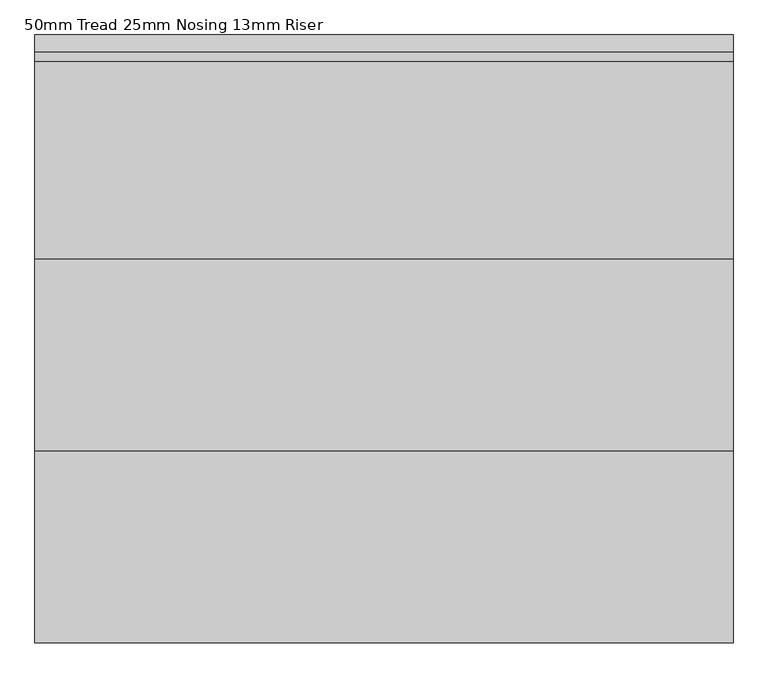
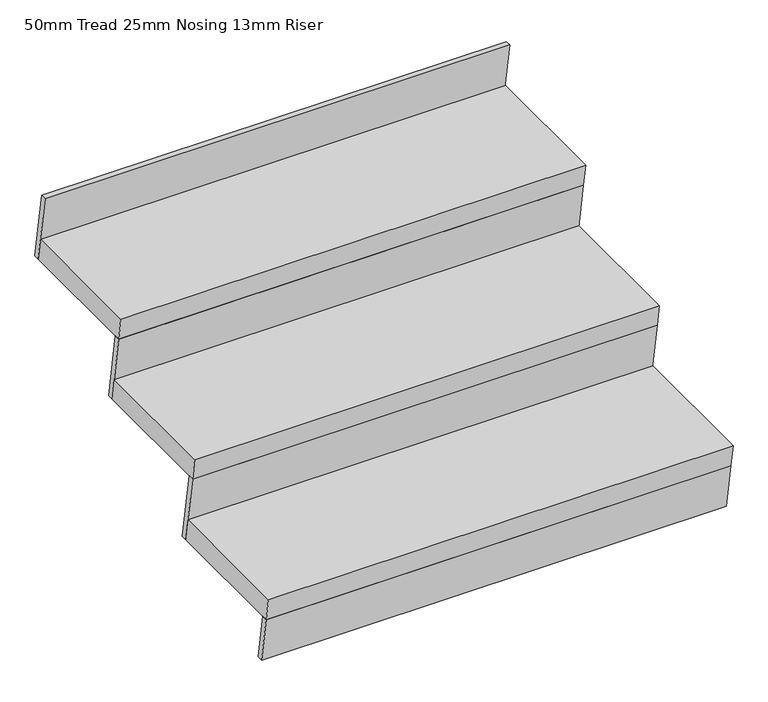
"""IFC4 building model written with IfcOpenShell, lengths in millimetres: stair flight geometry, 50mm Tread 25mm Nosing 13mm Riser."""

from ifc_helpers import new_model, si_unit, frame, origin, place, context, project, spatial, polyline, outline, extrude, source, transform, mapped, element, save


def stair_flight_50mm_tread_25mm_nosing_13mm_riser_f84e0c27(model_context):
    return source(origin(), model_context, "Body", "SweptSolid", [
        extrude(outline(polyline([(-5656.14356, -457.2), (-5356.14356, -457.2), (-5347.9414603, -507.2), (-5647.9414603, -507.2), (-5656.14356, -457.2)])), frame((-15773.6523905, 0.0, 0.0), z_axis=(1.0, 0.0, 0.0), x_axis=(0.0, 1.0, 0.0)), (0.0, 0.0, 1.0), 1000.0257813),
        extrude(outline(polyline([(-5647.9414603, -507.2), (-5635.2743907, -507.2), (-5618.4764904, -609.6), (-5631.14356, -609.6), (-5647.9414603, -507.2)])), frame((-15773.6523905, 0.0, 0.0), z_axis=(1.0, 0.0, 0.0), x_axis=(0.0, 1.0, 0.0)), (0.0, 0.0, 1.0), 1000.0257813),
        extrude(outline(polyline([(-5372.9414603, -354.8), (-5360.2743907, -354.8), (-5335.2743907, -507.2), (-5347.9414603, -507.2), (-5372.9414603, -354.8)])), frame((-15773.6523905, 0.0, 0.0), z_axis=(1.0, 0.0, 0.0), x_axis=(0.0, 1.0, 0.0)), (0.0, 0.0, 1.0), 1000.0257813),
        extrude(outline(polyline([(-5381.14356, -304.8), (-5081.14356, -304.8), (-5072.9414603, -354.8), (-5372.9414603, -354.8), (-5381.14356, -304.8)])), frame((-15773.6523905, 0.0, 0.0), z_axis=(1.0, 0.0, 0.0), x_axis=(0.0, 1.0, 0.0)), (0.0, 0.0, 1.0), 1000.0257813),
        extrude(outline(polyline([(-5097.9414603, -202.4), (-5085.2743907, -202.4), (-5060.2743907, -354.8), (-5072.9414603, -354.8), (-5097.9414603, -202.4)])), frame((-15773.6523905, 0.0, 0.0), z_axis=(1.0, 0.0, 0.0), x_axis=(0.0, 1.0, 0.0)), (0.0, 0.0, 1.0), 1000.0257813),
        extrude(outline(polyline([(-4822.9414603, -50.0), (-4810.2743907, -50.0), (-4785.2743907, -202.4), (-4797.9414603, -202.4), (-4822.9414603, -50.0)])), frame((-15773.6523905, 0.0, 0.0), z_axis=(1.0, 0.0, 0.0), x_axis=(0.0, 1.0, 0.0)), (0.0, 0.0, 1.0), 1000.0257813),
        extrude(outline(polyline([(-5106.14356, -152.4), (-4806.14356, -152.4), (-4797.9414603, -202.4), (-5097.9414603, -202.4), (-5106.14356, -152.4)])), frame((-15773.6523905, 0.0, 0.0), z_axis=(1.0, 0.0, 0.0), x_axis=(0.0, 1.0, 0.0)), (0.0, 0.0, 1.0), 1000.0257813),
    ])


if __name__ == "__main__":
    model = new_model("IFC4")
    model_context = context("Model", 3, world=origin())
    ifc_project = project(units=[si_unit("LENGTHUNIT", "METRE", prefix="MILLI")], contexts=[model_context])
    site = spatial("IfcSite", under=ifc_project)
    building = spatial("IfcBuilding", under=site)
    placement = place(None, origin())
    stair_flight_50mm_tread_25mm_nosing_13mm_riser_shape = stair_flight_50mm_tread_25mm_nosing_13mm_riser_f84e0c27(model_context)
    element("IfcStairFlight", 1, ObjectType="50mm Tread 25mm Nosing 13mm Riser", at=placement, inside=building, context=model_context, shape_type="MappedRepresentation", body=[
        mapped(stair_flight_50mm_tread_25mm_nosing_13mm_riser_shape, transform((0.0, 0.0, 0.0), x_axis=(1.0, 0.0, 0.0), y_axis=(0.0, 1.0, 0.0), z_axis=(0.0, 0.0, 1.0))),
    ])
    save(model, "model.ifc")
